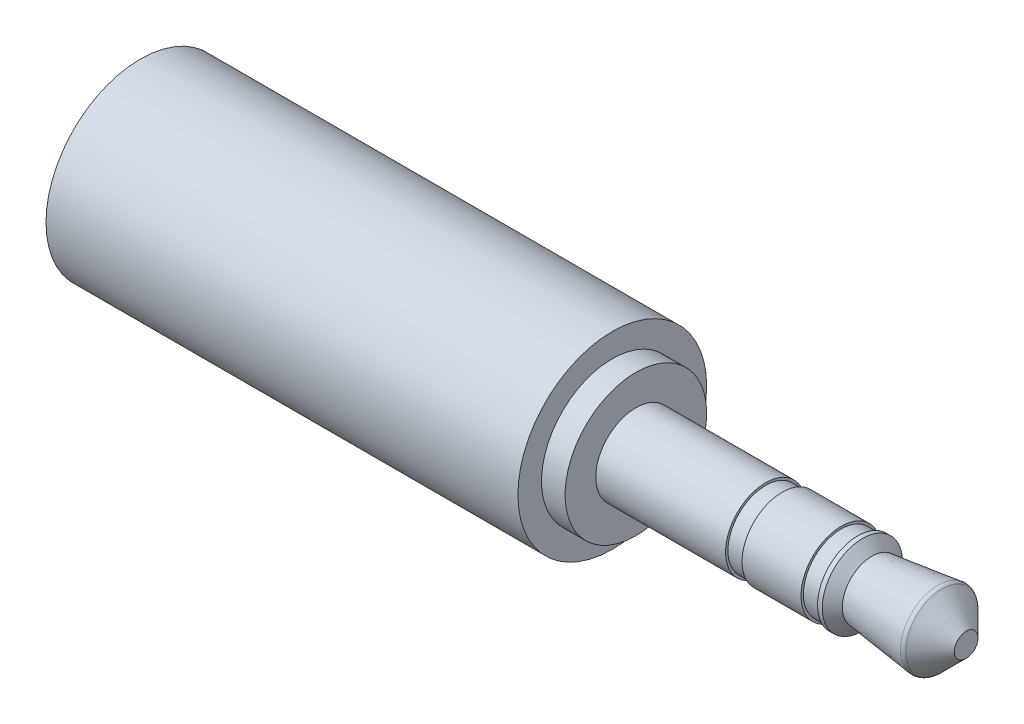
ISO-10303-21;
HEADER;
FILE_DESCRIPTION(('STEP AP214'),'2;1');
FILE_NAME('part.step','',(''),(''),'','','');
FILE_SCHEMA(('AUTOMOTIVE_DESIGN { 1 0 10303 214 1 1 1 1 }'));
ENDSEC;
DATA;
#1=APPLICATION_CONTEXT('core data for automotive mechanical design processes');
#2=APPLICATION_PROTOCOL_DEFINITION('international standard','automotive_design',2000,#1);
#3=PRODUCT_CONTEXT('',#1,'mechanical');
#4=PRODUCT('Part','Part','',(#3));
#5=PRODUCT_RELATED_PRODUCT_CATEGORY('part','',(#4));
#6=PRODUCT_DEFINITION_FORMATION('','',#4);
#7=PRODUCT_DEFINITION_CONTEXT('part definition',#1,'design');
#8=PRODUCT_DEFINITION('design','',#6,#7);
#9=PRODUCT_DEFINITION_SHAPE('','',#8);
#10=(LENGTH_UNIT() NAMED_UNIT(*) SI_UNIT(.MILLI.,.METRE.));
#11=(NAMED_UNIT(*) PLANE_ANGLE_UNIT() SI_UNIT($,.RADIAN.));
#12=(NAMED_UNIT(*) SI_UNIT($,.STERADIAN.) SOLID_ANGLE_UNIT());
#13=UNCERTAINTY_MEASURE_WITH_UNIT(LENGTH_MEASURE(1.E-05),#10,'distance_accuracy_value','');
#14=(GEOMETRIC_REPRESENTATION_CONTEXT(3) GLOBAL_UNCERTAINTY_ASSIGNED_CONTEXT((#13)) GLOBAL_UNIT_ASSIGNED_CONTEXT((#10,
#11,#12)) REPRESENTATION_CONTEXT('',''));
#15=CARTESIAN_POINT('',(0.,0.,0.));
#16=DIRECTION('',(0.,0.,1.));
#17=DIRECTION('',(1.,0.,0.));
#18=AXIS2_PLACEMENT_3D('',#15,#16,#17);
#19=CARTESIAN_POINT('',(0.,0.5,0.));
#20=DIRECTION('',(1.,0.,0.));
#21=DIRECTION('',(0.,0.,-1.));
#22=AXIS2_PLACEMENT_3D('',#19,#20,#21);
#23=PLANE('',#22);
#24=CARTESIAN_POINT('',(0.,0.,0.));
#25=DIRECTION('',(1.,0.,0.));
#26=DIRECTION('',(0.,0.,-1.));
#27=AXIS2_PLACEMENT_3D('',#24,#25,#26);
#28=CIRCLE('',#27,0.5);
#29=CARTESIAN_POINT('',(0.,0.,0.5));
#30=VERTEX_POINT('',#29);
#31=EDGE_CURVE('E96',#30,#30,#28,.T.);
#32=ORIENTED_EDGE('',*,*,#31,.T.);
#33=EDGE_LOOP('',(#32));
#34=FACE_BOUND('',#33,.T.);
#35=ADVANCED_FACE('F40',(#34),#23,.T.);
#36=CARTESIAN_POINT('',(-35.,0.,0.));
#37=DIRECTION('',(-1.,0.,0.));
#38=DIRECTION('',(0.,0.,1.));
#39=AXIS2_PLACEMENT_3D('',#36,#37,#38);
#40=PLANE('',#39);
#41=CARTESIAN_POINT('',(-35.,0.,0.));
#42=DIRECTION('',(1.,0.,0.));
#43=DIRECTION('',(0.,0.,-1.));
#44=AXIS2_PLACEMENT_3D('',#41,#42,#43);
#45=CIRCLE('',#44,4.);
#46=CARTESIAN_POINT('',(-35.,0.,-4.));
#47=VERTEX_POINT('',#46);
#48=EDGE_CURVE('E48',#47,#47,#45,.T.);
#49=ORIENTED_EDGE('',*,*,#48,.F.);
#50=EDGE_LOOP('',(#49));
#51=FACE_BOUND('',#50,.T.);
#52=ADVANCED_FACE('F114',(#51),#40,.T.);
#53=CARTESIAN_POINT('',(0.,0.,0.));
#54=DIRECTION('',(1.,0.,0.));
#55=DIRECTION('',(0.,0.,-1.));
#56=AXIS2_PLACEMENT_3D('',#53,#54,#55);
#57=CYLINDRICAL_SURFACE('',#56,4.);
#58=ORIENTED_EDGE('',*,*,#48,.T.);
#59=EDGE_LOOP('',(#58));
#60=FACE_BOUND('',#59,.T.);
#61=CARTESIAN_POINT('',(-15.,0.,0.));
#62=DIRECTION('',(1.,0.,0.));
#63=DIRECTION('',(0.,0.,-1.));
#64=AXIS2_PLACEMENT_3D('',#61,#62,#63);
#65=CIRCLE('',#64,4.);
#66=CARTESIAN_POINT('',(-15.,0.,-4.));
#67=VERTEX_POINT('',#66);
#68=EDGE_CURVE('E55',#67,#67,#65,.T.);
#69=ORIENTED_EDGE('',*,*,#68,.F.);
#70=EDGE_LOOP('',(#69));
#71=FACE_BOUND('',#70,.T.);
#72=ADVANCED_FACE('F116',(#60,#71),#57,.T.);
#73=CARTESIAN_POINT('',(-15.,4.,0.));
#74=DIRECTION('',(1.,0.,0.));
#75=DIRECTION('',(0.,0.,-1.));
#76=AXIS2_PLACEMENT_3D('',#73,#74,#75);
#77=PLANE('',#76);
#78=ORIENTED_EDGE('',*,*,#68,.T.);
#79=EDGE_LOOP('',(#78));
#80=FACE_BOUND('',#79,.T.);
#81=CARTESIAN_POINT('',(-15.,0.,0.));
#82=DIRECTION('',(1.,0.,0.));
#83=DIRECTION('',(0.,0.,-1.));
#84=AXIS2_PLACEMENT_3D('',#81,#82,#83);
#85=CIRCLE('',#84,3.);
#86=CARTESIAN_POINT('',(-15.,0.,-3.));
#87=VERTEX_POINT('',#86);
#88=EDGE_CURVE('E60',#87,#87,#85,.T.);
#89=ORIENTED_EDGE('',*,*,#88,.F.);
#90=EDGE_LOOP('',(#89));
#91=FACE_BOUND('',#90,.T.);
#92=ADVANCED_FACE('F124',(#80,#91),#77,.T.);
#93=CARTESIAN_POINT('',(0.,0.,0.));
#94=DIRECTION('',(1.,0.,0.));
#95=DIRECTION('',(0.,0.,-1.));
#96=AXIS2_PLACEMENT_3D('',#93,#94,#95);
#97=CYLINDRICAL_SURFACE('',#96,3.);
#98=ORIENTED_EDGE('',*,*,#88,.T.);
#99=EDGE_LOOP('',(#98));
#100=FACE_BOUND('',#99,.T.);
#101=CARTESIAN_POINT('',(-14.,0.,0.));
#102=DIRECTION('',(1.,0.,0.));
#103=DIRECTION('',(0.,0.,-1.));
#104=AXIS2_PLACEMENT_3D('',#101,#102,#103);
#105=CIRCLE('',#104,3.);
#106=CARTESIAN_POINT('',(-14.,0.,-3.));
#107=VERTEX_POINT('',#106);
#108=EDGE_CURVE('E58',#107,#107,#105,.T.);
#109=ORIENTED_EDGE('',*,*,#108,.F.);
#110=EDGE_LOOP('',(#109));
#111=FACE_BOUND('',#110,.T.);
#112=ADVANCED_FACE('F130',(#100,#111),#97,.T.);
#113=CARTESIAN_POINT('',(-14.,3.,0.));
#114=DIRECTION('',(1.,0.,0.));
#115=DIRECTION('',(0.,0.,-1.));
#116=AXIS2_PLACEMENT_3D('',#113,#114,#115);
#117=PLANE('',#116);
#118=ORIENTED_EDGE('',*,*,#108,.T.);
#119=EDGE_LOOP('',(#118));
#120=FACE_BOUND('',#119,.T.);
#121=CARTESIAN_POINT('',(-14.,0.,0.));
#122=DIRECTION('',(1.,0.,0.));
#123=DIRECTION('',(0.,0.,-1.));
#124=AXIS2_PLACEMENT_3D('',#121,#122,#123);
#125=CIRCLE('',#124,1.7);
#126=CARTESIAN_POINT('',(-14.,0.,-1.7));
#127=VERTEX_POINT('',#126);
#128=EDGE_CURVE('E65',#127,#127,#125,.T.);
#129=ORIENTED_EDGE('',*,*,#128,.F.);
#130=EDGE_LOOP('',(#129));
#131=FACE_BOUND('',#130,.T.);
#132=ADVANCED_FACE('F134',(#120,#131),#117,.T.);
#133=CARTESIAN_POINT('',(0.,0.,0.));
#134=DIRECTION('',(1.,0.,0.));
#135=DIRECTION('',(0.,0.,-1.));
#136=AXIS2_PLACEMENT_3D('',#133,#134,#135);
#137=CYLINDRICAL_SURFACE('',#136,1.7);
#138=ORIENTED_EDGE('',*,*,#128,.T.);
#139=EDGE_LOOP('',(#138));
#140=FACE_BOUND('',#139,.T.);
#141=CARTESIAN_POINT('',(-8.5,0.,0.));
#142=DIRECTION('',(1.,0.,0.));
#143=DIRECTION('',(0.,0.,-1.));
#144=AXIS2_PLACEMENT_3D('',#141,#142,#143);
#145=CIRCLE('',#144,1.7);
#146=CARTESIAN_POINT('',(-8.5,0.,-1.7));
#147=VERTEX_POINT('',#146);
#148=EDGE_CURVE('E67',#147,#147,#145,.T.);
#149=ORIENTED_EDGE('',*,*,#148,.F.);
#150=EDGE_LOOP('',(#149));
#151=FACE_BOUND('',#150,.T.);
#152=ADVANCED_FACE('F132',(#140,#151),#137,.T.);
#153=CARTESIAN_POINT('',(-8.5,1.7,0.));
#154=DIRECTION('',(1.,0.,0.));
#155=DIRECTION('',(0.,0.,-1.));
#156=AXIS2_PLACEMENT_3D('',#153,#154,#155);
#157=PLANE('',#156);
#158=ORIENTED_EDGE('',*,*,#148,.T.);
#159=EDGE_LOOP('',(#158));
#160=FACE_BOUND('',#159,.T.);
#161=CARTESIAN_POINT('',(-8.5,0.,0.));
#162=DIRECTION('',(1.,0.,0.));
#163=DIRECTION('',(0.,0.,-1.));
#164=AXIS2_PLACEMENT_3D('',#161,#162,#163);
#165=CIRCLE('',#164,1.6);
#166=CARTESIAN_POINT('',(-8.5,0.,-1.6));
#167=VERTEX_POINT('',#166);
#168=EDGE_CURVE('E66',#167,#167,#165,.T.);
#169=ORIENTED_EDGE('',*,*,#168,.F.);
#170=EDGE_LOOP('',(#169));
#171=FACE_BOUND('',#170,.T.);
#172=ADVANCED_FACE('F136',(#160,#171),#157,.T.);
#173=CARTESIAN_POINT('',(0.,0.,0.));
#174=DIRECTION('',(1.,0.,0.));
#175=DIRECTION('',(0.,0.,-1.));
#176=AXIS2_PLACEMENT_3D('',#173,#174,#175);
#177=CYLINDRICAL_SURFACE('',#176,1.6);
#178=ORIENTED_EDGE('',*,*,#168,.T.);
#179=EDGE_LOOP('',(#178));
#180=FACE_BOUND('',#179,.T.);
#181=CARTESIAN_POINT('',(-7.8,0.,0.));
#182=DIRECTION('',(1.,0.,0.));
#183=DIRECTION('',(0.,0.,-1.));
#184=AXIS2_PLACEMENT_3D('',#181,#182,#183);
#185=CIRCLE('',#184,1.6);
#186=CARTESIAN_POINT('',(-7.8,0.,-1.6));
#187=VERTEX_POINT('',#186);
#188=EDGE_CURVE('E75',#187,#187,#185,.T.);
#189=ORIENTED_EDGE('',*,*,#188,.F.);
#190=EDGE_LOOP('',(#189));
#191=FACE_BOUND('',#190,.T.);
#192=ADVANCED_FACE('F141',(#180,#191),#177,.T.);
#193=CARTESIAN_POINT('',(-7.8,1.6,0.));
#194=DIRECTION('',(-1.,0.,0.));
#195=DIRECTION('',(0.,0.,1.));
#196=AXIS2_PLACEMENT_3D('',#193,#194,#195);
#197=PLANE('',#196);
#198=ORIENTED_EDGE('',*,*,#188,.T.);
#199=EDGE_LOOP('',(#198));
#200=FACE_BOUND('',#199,.T.);
#201=CARTESIAN_POINT('',(-7.8,0.,0.));
#202=DIRECTION('',(1.,0.,0.));
#203=DIRECTION('',(0.,0.,-1.));
#204=AXIS2_PLACEMENT_3D('',#201,#202,#203);
#205=CIRCLE('',#204,1.7);
#206=CARTESIAN_POINT('',(-7.8,0.,-1.7));
#207=VERTEX_POINT('',#206);
#208=EDGE_CURVE('E73',#207,#207,#205,.T.);
#209=ORIENTED_EDGE('',*,*,#208,.F.);
#210=EDGE_LOOP('',(#209));
#211=FACE_BOUND('',#210,.T.);
#212=ADVANCED_FACE('F150',(#200,#211),#197,.T.);
#213=CARTESIAN_POINT('',(0.,0.,0.));
#214=DIRECTION('',(1.,0.,0.));
#215=DIRECTION('',(0.,0.,-1.));
#216=AXIS2_PLACEMENT_3D('',#213,#214,#215);
#217=CYLINDRICAL_SURFACE('',#216,1.7);
#218=ORIENTED_EDGE('',*,*,#208,.T.);
#219=EDGE_LOOP('',(#218));
#220=FACE_BOUND('',#219,.T.);
#221=CARTESIAN_POINT('',(-5.3,0.,0.));
#222=DIRECTION('',(1.,0.,0.));
#223=DIRECTION('',(0.,0.,-1.));
#224=AXIS2_PLACEMENT_3D('',#221,#222,#223);
#225=CIRCLE('',#224,1.7);
#226=CARTESIAN_POINT('',(-5.3,0.,-1.7));
#227=VERTEX_POINT('',#226);
#228=EDGE_CURVE('E80',#227,#227,#225,.T.);
#229=ORIENTED_EDGE('',*,*,#228,.F.);
#230=EDGE_LOOP('',(#229));
#231=FACE_BOUND('',#230,.T.);
#232=ADVANCED_FACE('F151',(#220,#231),#217,.T.);
#233=CARTESIAN_POINT('',(-5.3,1.7,0.));
#234=DIRECTION('',(1.,0.,0.));
#235=DIRECTION('',(0.,0.,-1.));
#236=AXIS2_PLACEMENT_3D('',#233,#234,#235);
#237=PLANE('',#236);
#238=ORIENTED_EDGE('',*,*,#228,.T.);
#239=EDGE_LOOP('',(#238));
#240=FACE_BOUND('',#239,.T.);
#241=CARTESIAN_POINT('',(-5.3,0.,0.));
#242=DIRECTION('',(1.,0.,0.));
#243=DIRECTION('',(0.,0.,-1.));
#244=AXIS2_PLACEMENT_3D('',#241,#242,#243);
#245=CIRCLE('',#244,1.6);
#246=CARTESIAN_POINT('',(-5.3,0.,-1.6));
#247=VERTEX_POINT('',#246);
#248=EDGE_CURVE('E82',#247,#247,#245,.T.);
#249=ORIENTED_EDGE('',*,*,#248,.F.);
#250=EDGE_LOOP('',(#249));
#251=FACE_BOUND('',#250,.T.);
#252=ADVANCED_FACE('F154',(#240,#251),#237,.T.);
#253=CARTESIAN_POINT('',(0.,0.,0.));
#254=DIRECTION('',(1.,0.,0.));
#255=DIRECTION('',(0.,0.,-1.));
#256=AXIS2_PLACEMENT_3D('',#253,#254,#255);
#257=CYLINDRICAL_SURFACE('',#256,1.6);
#258=ORIENTED_EDGE('',*,*,#248,.T.);
#259=EDGE_LOOP('',(#258));
#260=FACE_BOUND('',#259,.T.);
#261=CARTESIAN_POINT('',(-4.6,0.,0.));
#262=DIRECTION('',(1.,0.,0.));
#263=DIRECTION('',(0.,0.,-1.));
#264=AXIS2_PLACEMENT_3D('',#261,#262,#263);
#265=CIRCLE('',#264,1.6);
#266=CARTESIAN_POINT('',(-4.6,0.,-1.6));
#267=VERTEX_POINT('',#266);
#268=EDGE_CURVE('E81',#267,#267,#265,.T.);
#269=ORIENTED_EDGE('',*,*,#268,.F.);
#270=EDGE_LOOP('',(#269));
#271=FACE_BOUND('',#270,.T.);
#272=ADVANCED_FACE('F157',(#260,#271),#257,.T.);
#273=CARTESIAN_POINT('',(-4.6,1.6,0.));
#274=DIRECTION('',(-1.,0.,0.));
#275=DIRECTION('',(0.,0.,1.));
#276=AXIS2_PLACEMENT_3D('',#273,#274,#275);
#277=PLANE('',#276);
#278=ORIENTED_EDGE('',*,*,#268,.T.);
#279=EDGE_LOOP('',(#278));
#280=FACE_BOUND('',#279,.T.);
#281=CARTESIAN_POINT('',(-4.6,0.,0.));
#282=DIRECTION('',(1.,0.,0.));
#283=DIRECTION('',(0.,0.,-1.));
#284=AXIS2_PLACEMENT_3D('',#281,#282,#283);
#285=CIRCLE('',#284,1.7);
#286=CARTESIAN_POINT('',(-4.6,0.,-1.7));
#287=VERTEX_POINT('',#286);
#288=EDGE_CURVE('E87',#287,#287,#285,.T.);
#289=ORIENTED_EDGE('',*,*,#288,.F.);
#290=EDGE_LOOP('',(#289));
#291=FACE_BOUND('',#290,.T.);
#292=ADVANCED_FACE('F162',(#280,#291),#277,.T.);
#293=CARTESIAN_POINT('',(0.,0.,0.));
#294=DIRECTION('',(1.,0.,0.));
#295=DIRECTION('',(0.,0.,-1.));
#296=AXIS2_PLACEMENT_3D('',#293,#294,#295);
#297=CYLINDRICAL_SURFACE('',#296,1.7);
#298=ORIENTED_EDGE('',*,*,#288,.T.);
#299=EDGE_LOOP('',(#298));
#300=FACE_BOUND('',#299,.T.);
#301=CARTESIAN_POINT('',(-4.4,0.,0.));
#302=DIRECTION('',(1.,0.,0.));
#303=DIRECTION('',(0.,0.,-1.));
#304=AXIS2_PLACEMENT_3D('',#301,#302,#303);
#305=CIRCLE('',#304,1.7);
#306=CARTESIAN_POINT('',(-4.4,0.,-1.7));
#307=VERTEX_POINT('',#306);
#308=EDGE_CURVE('E89',#307,#307,#305,.T.);
#309=ORIENTED_EDGE('',*,*,#308,.F.);
#310=EDGE_LOOP('',(#309));
#311=FACE_BOUND('',#310,.T.);
#312=ADVANCED_FACE('F170',(#300,#311),#297,.T.);
#313=CARTESIAN_POINT('',(-4.,0.,0.));
#314=DIRECTION('',(-1.,0.,0.));
#315=DIRECTION('',(0.,0.,1.));
#316=AXIS2_PLACEMENT_3D('',#313,#314,#315);
#317=CONICAL_SURFACE('',#316,1.25,0.844153986113166);
#318=ORIENTED_EDGE('',*,*,#308,.T.);
#319=EDGE_LOOP('',(#318));
#320=FACE_BOUND('',#319,.T.);
#321=CARTESIAN_POINT('',(-4.,0.,0.));
#322=DIRECTION('',(1.,0.,0.));
#323=DIRECTION('',(0.,0.,-1.));
#324=AXIS2_PLACEMENT_3D('',#321,#322,#323);
#325=CIRCLE('',#324,1.25);
#326=CARTESIAN_POINT('',(-4.,0.,-1.25));
#327=VERTEX_POINT('',#326);
#328=EDGE_CURVE('E91',#327,#327,#325,.T.);
#329=ORIENTED_EDGE('',*,*,#328,.F.);
#330=EDGE_LOOP('',(#329));
#331=FACE_BOUND('',#330,.T.);
#332=ADVANCED_FACE('F109',(#320,#331),#317,.T.);
#333=CARTESIAN_POINT('',(-1.1,0.,0.));
#334=DIRECTION('',(1.,0.,0.));
#335=DIRECTION('',(0.,0.,-1.));
#336=AXIS2_PLACEMENT_3D('',#333,#334,#335);
#337=CONICAL_SURFACE('',#336,1.6,0.120108735566913);
#338=CARTESIAN_POINT('',(-1.19659018570502,0.,0.));
#339=DIRECTION('',(-1.,0.,0.));
#340=DIRECTION('',(0.,0.,1.));
#341=AXIS2_PLACEMENT_3D('',#338,#339,#340);
#342=CIRCLE('',#341,1.58834256379422);
#343=CARTESIAN_POINT('',(-1.19659018570502,0.,1.58834256379422));
#344=VERTEX_POINT('',#343);
#345=EDGE_CURVE('E10',#344,#344,#342,.T.);
#346=ORIENTED_EDGE('',*,*,#345,.T.);
#347=EDGE_LOOP('',(#346));
#348=FACE_BOUND('',#347,.T.);
#349=ORIENTED_EDGE('',*,*,#328,.T.);
#350=EDGE_LOOP('',(#349));
#351=FACE_BOUND('',#350,.T.);
#352=ADVANCED_FACE('F103',(#348,#351),#337,.T.);
#353=CARTESIAN_POINT('',(0.,0.,0.));
#354=DIRECTION('',(-1.,0.,0.));
#355=DIRECTION('',(0.,0.,1.));
#356=AXIS2_PLACEMENT_3D('',#353,#354,#355);
#357=CONICAL_SURFACE('',#356,0.5,0.785398163397446);
#358=CARTESIAN_POINT('',(-1.03120479742954,0.,0.));
#359=DIRECTION('',(1.,0.,0.));
#360=DIRECTION('',(0.,0.,-1.));
#361=AXIS2_PLACEMENT_3D('',#358,#359,#360);
#362=CIRCLE('',#361,1.53120479742954);
#363=CARTESIAN_POINT('',(-1.03120479742954,0.,1.53120479742954));
#364=VERTEX_POINT('',#363);
#365=EDGE_CURVE('E42',#364,#364,#362,.T.);
#366=CARTESIAN_POINT('',(-1.03120479742954,0.,1.53120479742954));
#367=CARTESIAN_POINT('',(-1.02046308078965,0.,1.52046308078965));
#368=CARTESIAN_POINT('',(-1.00972136414976,0.,1.50972136414976));
#369=CARTESIAN_POINT('',(-0.988237930869978,0.,1.48823793086997));
#370=CARTESIAN_POINT('',(-0.977496214230087,0.,1.47749621423008));
#371=CARTESIAN_POINT('',(-0.956012780950305,0.,1.4560127809503));
#372=CARTESIAN_POINT('',(-0.945271064310414,0.,1.44527106431041));
#373=CARTESIAN_POINT('',(-0.923787631030632,0.,1.42378763103063));
#374=CARTESIAN_POINT('',(-0.913045914390741,0.,1.41304591439074));
#375=CARTESIAN_POINT('',(-0.891562481110958,0.,1.39156248111096));
#376=CARTESIAN_POINT('',(-0.880820764471067,0.,1.38082076447106));
#377=CARTESIAN_POINT('',(-0.859337331191285,0.,1.35933733119128));
#378=CARTESIAN_POINT('',(-0.848595614551394,0.,1.34859561455139));
#379=CARTESIAN_POINT('',(-0.827112181271612,0.,1.32711218127161));
#380=CARTESIAN_POINT('',(-0.816370464631721,0.,1.31637046463172));
#381=CARTESIAN_POINT('',(-0.794887031351939,0.,1.29488703135194));
#382=CARTESIAN_POINT('',(-0.784145314712048,0.,1.28414531471204));
#383=CARTESIAN_POINT('',(-0.762661881432266,0.,1.26266188143226));
#384=CARTESIAN_POINT('',(-0.751920164792375,0.,1.25192016479237));
#385=CARTESIAN_POINT('',(-0.730436731512592,0.,1.23043673151259));
#386=CARTESIAN_POINT('',(-0.719695014872701,0.,1.2196950148727));
#387=CARTESIAN_POINT('',(-0.698211581592919,0.,1.19821158159292));
#388=CARTESIAN_POINT('',(-0.687469864953028,0.,1.18746986495303));
#389=CARTESIAN_POINT('',(-0.665986431673246,0.,1.16598643167324));
#390=CARTESIAN_POINT('',(-0.655244715033355,0.,1.15524471503335));
#391=CARTESIAN_POINT('',(-0.633761281753573,0.,1.13376128175357));
#392=CARTESIAN_POINT('',(-0.623019565113682,0.,1.12301956511368));
#393=CARTESIAN_POINT('',(-0.6015361318339,0.,1.1015361318339));
#394=CARTESIAN_POINT('',(-0.590794415194009,0.,1.09079441519401));
#395=CARTESIAN_POINT('',(-0.569310981914226,0.,1.06931098191422));
#396=CARTESIAN_POINT('',(-0.558569265274335,0.,1.05856926527433));
#397=CARTESIAN_POINT('',(-0.537085831994553,0.,1.03708583199455));
#398=CARTESIAN_POINT('',(-0.526344115354662,0.,1.02634411535466));
#399=CARTESIAN_POINT('',(-0.50486068207488,0.,1.00486068207488));
#400=CARTESIAN_POINT('',(-0.494118965434989,0.,0.994118965434987));
#401=CARTESIAN_POINT('',(-0.472635532155207,0.,0.972635532155205));
#402=CARTESIAN_POINT('',(-0.461893815515316,0.,0.961893815515314));
#403=CARTESIAN_POINT('',(-0.440410382235534,0.,0.940410382235532));
#404=CARTESIAN_POINT('',(-0.429668665595643,0.,0.929668665595641));
#405=CARTESIAN_POINT('',(-0.40818523231586,0.,0.908185232315859));
#406=CARTESIAN_POINT('',(-0.397443515675969,0.,0.897443515675968));
#407=CARTESIAN_POINT('',(-0.375960082396187,0.,0.875960082396186));
#408=CARTESIAN_POINT('',(-0.365218365756296,0.,0.865218365756295));
#409=CARTESIAN_POINT('',(-0.343734932476514,0.,0.843734932476513));
#410=CARTESIAN_POINT('',(-0.332993215836623,0.,0.832993215836622));
#411=CARTESIAN_POINT('',(-0.311509782556841,0.,0.81150978255684));
#412=CARTESIAN_POINT('',(-0.30076806591695,0.,0.800768065916949));
#413=CARTESIAN_POINT('',(-0.279284632637168,0.,0.779284632637167));
#414=CARTESIAN_POINT('',(-0.268542915997277,0.,0.768542915997276));
#415=CARTESIAN_POINT('',(-0.247059482717494,0.,0.747059482717493));
#416=CARTESIAN_POINT('',(-0.236317766077603,0.,0.736317766077602));
#417=CARTESIAN_POINT('',(-0.214834332797821,0.,0.71483433279782));
#418=CARTESIAN_POINT('',(-0.20409261615793,0.,0.704092616157929));
#419=CARTESIAN_POINT('',(-0.182609182878148,0.,0.682609182878147));
#420=CARTESIAN_POINT('',(-0.171867466238257,0.,0.671867466238256));
#421=CARTESIAN_POINT('',(-0.150384032958475,0.,0.650384032958474));
#422=CARTESIAN_POINT('',(-0.139642316318584,0.,0.639642316318583));
#423=CARTESIAN_POINT('',(-0.118158883038802,0.,0.618158883038801));
#424=CARTESIAN_POINT('',(-0.107417166398911,0.,0.60741716639891));
#425=CARTESIAN_POINT('',(-0.0859337331191284,0.,0.585933733119128));
#426=CARTESIAN_POINT('',(-0.0751920164792373,0.,0.575192016479237));
#427=CARTESIAN_POINT('',(-0.0537085831994552,0.,0.553708583199455));
#428=CARTESIAN_POINT('',(-0.0429668665595641,0.,0.542966866559564));
#429=CARTESIAN_POINT('',(-0.0214834332797819,0.,0.521483433279782));
#430=CARTESIAN_POINT('',(-0.0107417166398909,0.,0.510741716639891));
#431=CARTESIAN_POINT('',(0.,0.,0.5));
#432=B_SPLINE_CURVE_WITH_KNOTS('',3,(#366,#367,#368,#369,#370,#371,#372,#373,#374,#375,#376,
#377,#378,#379,#380,#381,#382,#383,#384,#385,#386,#387,#388,#389,#390,#391,#392,#393,#394,#395,
#396,#397,#398,#399,#400,#401,#402,#403,#404,#405,#406,#407,#408,#409,#410,#411,#412,#413,#414,
#415,#416,#417,#418,#419,#420,#421,#422,#423,#424,#425,#426,#427,#428,#429,#430,#431),
.UNSPECIFIED.,.F.,.F.,(4,2,2,2,2,2,2,2,2,2,2,2,2,2,2,2,2,2,2,2,2,2,2,2,2,2,2,2,2,2,2,2,4),(0.,
0.0455732440659078,0.0911464881318161,0.136719732197724,0.182292976263632,0.22786622032954,
0.273439464395448,0.319012708461356,0.364585952527264,0.410159196593172,0.45573244065908,
0.501305684724988,0.546878928790896,0.592452172856804,0.638025416922712,0.68359866098862,
0.729171905054528,0.774745149120436,0.820318393186344,0.865891637252252,0.91146488131816,
0.957038125384068,1.00261136944998,1.04818461351588,1.09375785758179,1.1393311016477,
1.18490434571361,1.23047758977952,1.27605083384542,1.32162407791133,1.36719732197724,
1.41277056604315,1.45834381010906),.UNSPECIFIED.);
#433=EDGE_CURVE('BSEAM101',#364,#30,#432,.T.);
#434=ORIENTED_EDGE('',*,*,#365,.T.);
#435=ORIENTED_EDGE('',*,*,#31,.F.);
#436=ORIENTED_EDGE('',*,*,#433,.T.);
#437=ORIENTED_EDGE('',*,*,#433,.F.);
#438=EDGE_LOOP('',(#434,#436,#435,#437));
#439=FACE_BOUND('',#438,.T.);
#440=ADVANCED_FACE('F101',(#439),#357,.T.);
#441=CARTESIAN_POINT('',(-1.17262615366685,0.,0.));
#442=DIRECTION('',(-1.,0.,0.));
#443=DIRECTION('',(0.,0.,1.));
#444=AXIS2_PLACEMENT_3D('',#441,#442,#443);
#445=TOROIDAL_SURFACE('',#444,1.38978344119223,0.2);
#446=ORIENTED_EDGE('',*,*,#345,.F.);
#447=EDGE_LOOP('',(#446));
#448=FACE_BOUND('',#447,.T.);
#449=ORIENTED_EDGE('',*,*,#365,.F.);
#450=EDGE_LOOP('',(#449));
#451=FACE_BOUND('',#450,.T.);
#452=ADVANCED_FACE('F39',(#448,#451),#445,.T.);
#453=CLOSED_SHELL('',(#35,#52,#72,#92,#112,#132,#152,#172,#192,#212,#232,#252,#272,#292,#312,
#332,#352,#440,#452));
#454=MANIFOLD_SOLID_BREP('B2',#453);
#455=ADVANCED_BREP_SHAPE_REPRESENTATION('',(#18,#454),#14);
#456=SHAPE_DEFINITION_REPRESENTATION(#9,#455);
ENDSEC;
END-ISO-10303-21;
